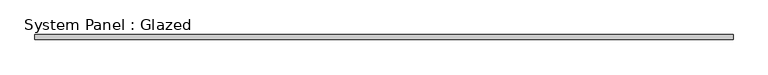
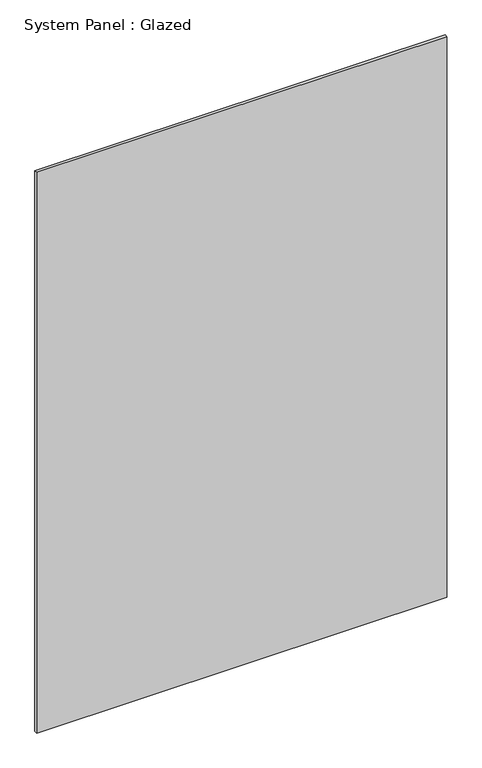
"""IFC4 building model written with IfcOpenShell, lengths in millimetres: plate geometry, System Panel : Glazed."""

from ifc_helpers import new_model, si_unit, origin, origin_with_axes, place, context, project, spatial, polyline, outline, extrude, source, transform, mapped, element, save


def system_panel_glazed_2aedba99(model_context):
    return source(origin(), model_context, "Body", "SweptSolid", [
        extrude(outline(polyline([(1749.2775428, 19.05), (-1749.2775428, 19.05), (-1749.2775428, 44.45), (1749.2775428, 44.45), (1749.2775428, 19.05)])), origin_with_axes(), (0.0, 0.0, 1.0), 5054.6),
    ])


if __name__ == "__main__":
    model = new_model("IFC4")
    model_context = context("Model", 3, world=origin())
    ifc_project = project(units=[si_unit("LENGTHUNIT", "METRE", prefix="MILLI")], contexts=[model_context])
    site = spatial("IfcSite", under=ifc_project)
    building = spatial("IfcBuilding", under=site)
    placement = place(None, origin())
    system_panel_glazed_shape = system_panel_glazed_2aedba99(model_context)
    element("IfcPlate", 1, ObjectType="System Panel : Glazed", at=placement, inside=building, context=model_context, shape_type="MappedRepresentation", body=[
        mapped(system_panel_glazed_shape, transform((0.0, 0.0, 0.0), x_axis=(1.0, 0.0, 0.0), y_axis=(0.0, 1.0, 0.0), z_axis=(0.0, 0.0, 1.0))),
    ])
    save(model, "model.ifc")

# Revit data of these elements
# Type "System Panel : Glazed"
#   Construction Type Id = "GSP4R"
#   Analytic Construction = "1/8 in Pilkington single glazing"
#   Visual Light Transmittance = 0.9
#   Solar Heat Gain Coefficient = 0.86
#   Heat Transfer Coefficient (U) = 1.18115 BTU/(h·ft²·°F)
# Element 1 (IfcPlate, "System Panel : Glazed")
#   Materials on its faces: "Glass"
# Materials
#   "Glass": class "Glass", colour RGB 0 128 192, transparency 0.75, Description = "Soda Lime Glass", Cost = 0
